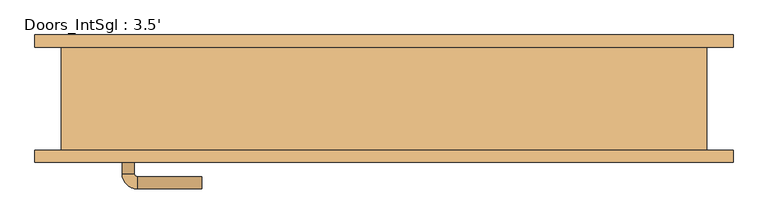
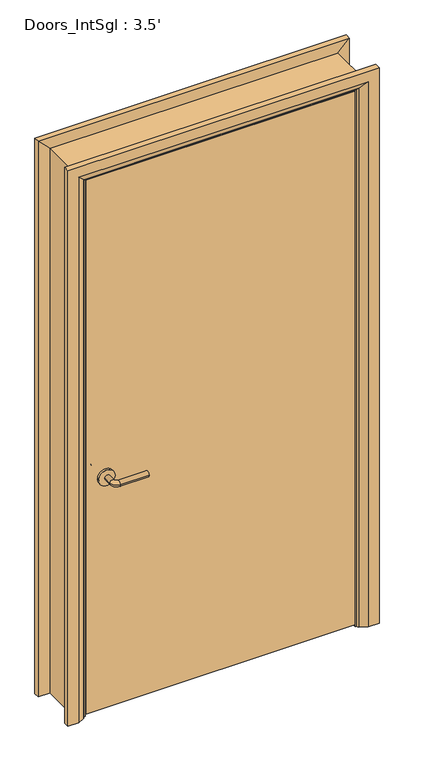
"""IFC4 building model written with IfcOpenShell, lengths in millimetres: door geometry, Doors_IntSgl : 3.5'."""

from ifc_helpers import new_model, si_unit, point, frame, frame_2d, origin, place, context, project, spatial, polyline, circle_curve, ellipse_curve, trimmed, segment, composite_curve, outline, extrude, faceted_brep, source, transform, mapped, element, save
from ifc_brep_helpers import plane_surface, cylinder_surface, revolved_surface, advanced_brep


def doors_intsgl_3_5_a4e1cc10(model_context):
    return source(origin(), model_context, "Body", "SolidModel", [
        advanced_brep(
        [(-426.4, -37.82, 900.0), (-406.4, -37.82, 900.0), (-426.4, -7.82, 900.0), (-406.4, -7.82, 900.0), (-401.4, -2.82, 900.0), (-401.4, 17.18, 900.0), (-296.4, 17.18, 900.0), (-296.4, -2.82, 900.0)],
        [
            (0, 1, circle_curve(frame((-416.4, -37.82, 900.0), z_axis=(0.0, -1.0, 0.0), x_axis=(1.0, 0.0, 0.0)), 10.0)),
            (1, 0, circle_curve(frame((-416.4, -37.82, 900.0), z_axis=(0.0, -1.0, 0.0), x_axis=(1.0, 0.0, 0.0)), 10.0)),
            (0, 2),
            (2, 3, circle_curve(frame((-416.4, -7.82, 900.0), z_axis=(0.0, -1.0, 0.0), x_axis=(1.0, 0.0, 0.0)), 10.0)),
            (3, 1),
            (3, 2, circle_curve(frame((-416.4, -7.82, 900.0), z_axis=(0.0, -1.0, 0.0), x_axis=(1.0, 0.0, 0.0)), 10.0)),
            (4, 3, circle_curve(frame((-401.4, -7.82, 900.0), z_axis=(0.0, 0.0, 1.0), x_axis=(-1.0, 0.0, 0.0)), 5.0)),
            (2, 5, circle_curve(frame((-401.4, -7.82, 900.0), z_axis=(0.0, 0.0, -1.0), x_axis=(-1.0, 0.0, 0.0)), 25.0)),
            (5, 4, circle_curve(frame((-401.4, 7.18, 900.0), z_axis=(-1.0, 0.0, 0.0), x_axis=(0.0, -1.0, 0.0)), 10.0)),
            (4, 5, circle_curve(frame((-401.4, 7.18, 900.0), z_axis=(-1.0, 0.0, 0.0), x_axis=(0.0, -1.0, 0.0)), 10.0)),
            (6, 7, circle_curve(frame((-296.4, 7.18, 900.0), z_axis=(1.0, 0.0, 0.0), x_axis=(0.0, -1.0, 0.0)), 10.0)),
            (7, 6, circle_curve(frame((-296.4, 7.18, 900.0), z_axis=(1.0, 0.0, 0.0), x_axis=(0.0, -1.0, 0.0)), 10.0)),
            (5, 6),
            (7, 4),
        ],
        [
            plane_surface(frame((-416.4, -37.82, 900.0), z_axis=(0.0, -1.0, 0.0), x_axis=(0.0, 0.0, 1.0))),
            cylinder_surface(frame((-416.4, -37.82, 900.0), z_axis=(0.0, -1.0, 0.0), x_axis=(1.0, 0.0, 0.0)), 10.0),
            revolved_surface(trimmed(ellipse_curve(frame((-416.4, -7.82, 900.0), z_axis=(0.0, -1.0, 0.0), x_axis=(1.0, 0.0, 0.0)), 10.0, 10.0), [point((-426.4, -7.82, 900.0))], [point((-406.4, -7.82, 900.0))], True, "CARTESIAN"), (-401.4, -7.82, 900.0), (0.0, 0.0, -1.0)),
            revolved_surface(trimmed(ellipse_curve(frame((-416.4, -7.82, 900.0), z_axis=(0.0, -1.0, 0.0), x_axis=(1.0, 0.0, 0.0)), 10.0, 10.0), [point((-406.4, -7.82, 900.0))], [point((-426.4, -7.82, 900.0))], True, "CARTESIAN"), (-401.4, -7.82, 900.0), (0.0, 0.0, -1.0)),
            plane_surface(frame((-296.4, 7.18, 900.0), z_axis=(1.0, 0.0, 0.0), x_axis=(0.0, 0.0, 1.0))),
            cylinder_surface(frame((-401.4, 7.18, 900.0), z_axis=(-1.0, 0.0, 0.0), x_axis=(0.0, -1.0, 0.0)), 10.0),
        ],
        [
            (0, [[1, 2]]),
            (1, [[-1, 3, 4, 5]]),
            (1, [[-2, -5, 6, -3]]),
            (2, [[7, -4, 8, 9]]),
            (3, [[-8, -6, -7, 10]]),
            (4, [[11, 12]]),
            (5, [[-9, 13, -12, 14]]),
            (5, [[-10, -14, -11, -13]]),
        ],
    ),
        extrude(outline(composite_curve([segment(trimmed(circle_curve(frame_2d((900.0, -418.9)), 30.0), [point((900.0, -448.9))], [point((900.0, -388.9))], False, "CARTESIAN"), True, "CONTINUOUS"), segment(trimmed(circle_curve(frame_2d((900.0, -418.9)), 30.0), [point((900.0, -388.9))], [point((900.0, -448.9))], False, "CARTESIAN"), True, "CONTINUOUS")], self_intersect=False)), frame((0.0, -45.82, 0.0), z_axis=(0.0, 1.0, 0.0), x_axis=(0.0, 0.0, 1.0)), (0.0, 0.0, 1.0), 8.0),
        advanced_brep(
        [(-426.4, -91.82, 900.0), (-406.4, -91.82, 900.0), (-406.4, -121.82, 900.0), (-426.4, -121.82, 900.0), (-401.4, -126.82, 900.0), (-401.4, -146.82, 900.0), (-296.4, -146.82, 900.0), (-296.4, -126.82, 900.0)],
        [
            (0, 1, circle_curve(frame((-416.4, -91.82, 900.0), z_axis=(0.0, 1.0, 0.0), x_axis=(1.0, 0.0, 0.0)), 10.0)),
            (1, 0, circle_curve(frame((-416.4, -91.82, 900.0), z_axis=(0.0, 1.0, 0.0), x_axis=(1.0, 0.0, 0.0)), 10.0)),
            (1, 2),
            (2, 3, circle_curve(frame((-416.4, -121.82, 900.0), z_axis=(0.0, 1.0, 0.0), x_axis=(1.0, 0.0, 0.0)), 10.0)),
            (3, 0),
            (3, 2, circle_curve(frame((-416.4, -121.82, 900.0), z_axis=(0.0, 1.0, 0.0), x_axis=(1.0, 0.0, 0.0)), 10.0)),
            (4, 5, circle_curve(frame((-401.4, -136.82, 900.0), z_axis=(-1.0, 0.0, 0.0), x_axis=(0.0, 1.0, 0.0)), 10.0)),
            (5, 3, circle_curve(frame((-401.4, -121.82, 900.0), z_axis=(0.0, 0.0, -1.0), x_axis=(-1.0, 0.0, 0.0)), 25.0)),
            (2, 4, circle_curve(frame((-401.4, -121.82, 900.0), z_axis=(0.0, 0.0, 1.0), x_axis=(-1.0, 0.0, 0.0)), 5.0)),
            (5, 4, circle_curve(frame((-401.4, -136.82, 900.0), z_axis=(-1.0, 0.0, 0.0), x_axis=(0.0, 1.0, 0.0)), 10.0)),
            (6, 7, circle_curve(frame((-296.4, -136.82, 900.0), z_axis=(1.0, 0.0, 0.0), x_axis=(0.0, 1.0, 0.0)), 10.0)),
            (7, 6, circle_curve(frame((-296.4, -136.82, 900.0), z_axis=(1.0, 0.0, 0.0), x_axis=(0.0, 1.0, 0.0)), 10.0)),
            (4, 7),
            (6, 5),
        ],
        [
            plane_surface(frame((-416.4, -91.82, 900.0), z_axis=(0.0, 1.0, 0.0), x_axis=(0.0, 0.0, 1.0))),
            cylinder_surface(frame((-416.4, -91.82, 900.0), z_axis=(0.0, 1.0, 0.0), x_axis=(1.0, 0.0, 0.0)), 10.0),
            revolved_surface(trimmed(ellipse_curve(frame((-416.4, -121.82, 900.0), z_axis=(0.0, -1.0, 0.0), x_axis=(1.0, 0.0, 0.0)), 10.0, 10.0), [point((-426.4, -121.82, 900.0))], [point((-406.4, -121.82, 900.0))], True, "CARTESIAN"), (-401.4, -121.82, 900.0), (0.0, 0.0, -1.0)),
            revolved_surface(trimmed(ellipse_curve(frame((-416.4, -121.82, 900.0), z_axis=(0.0, -1.0, 0.0), x_axis=(1.0, 0.0, 0.0)), 10.0, 10.0), [point((-406.4, -121.82, 900.0))], [point((-426.4, -121.82, 900.0))], True, "CARTESIAN"), (-401.4, -121.82, 900.0), (0.0, 0.0, -1.0)),
            plane_surface(frame((-296.4, -136.82, 900.0), z_axis=(1.0, 0.0, 0.0), x_axis=(0.0, 0.0, 1.0))),
            cylinder_surface(frame((-401.4, -136.82, 900.0), z_axis=(-1.0, 0.0, 0.0), x_axis=(0.0, 1.0, 0.0)), 10.0),
        ],
        [
            (0, [[1, 2]]),
            (1, [[3, 4, 5, -2]]),
            (1, [[-5, 6, -3, -1]]),
            (2, [[7, 8, -4, 9]]),
            (3, [[10, -9, -6, -8]]),
            (4, [[11, 12]]),
            (5, [[13, -11, 14, -7]]),
            (5, [[-14, -12, -13, -10]]),
        ],
    ),
        extrude(outline(composite_curve([segment(trimmed(circle_curve(frame_2d((900.0, -418.9)), 30.0), [point((900.0, -448.9))], [point((900.0, -388.9))], False, "CARTESIAN"), True, "CONTINUOUS"), segment(trimmed(circle_curve(frame_2d((900.0, -418.9)), 30.0), [point((900.0, -388.9))], [point((900.0, -448.9))], False, "CARTESIAN"), True, "CONTINUOUS")], self_intersect=False)), frame((0.0, -91.82, 0.0), z_axis=(0.0, 1.0, 0.0), x_axis=(0.0, 0.0, 1.0)), (0.0, 0.0, 1.0), 8.0),
        extrude(outline(polyline([(491.4, -45.82), (491.4, -83.82), (-491.4, -83.82), (-491.4, -45.82), (491.4, -45.82)])), frame((0.0, 0.0, 8.0), z_axis=(0.0, 0.0, 1.0), x_axis=(1.0, 0.0, 0.0)), (0.0, 0.0, 1.0), 2060.0),
        advanced_brep(
        [(568.4, -103.82, 0.0), (528.4, -103.82, 0.0), (502.4, -89.82, 0.0), (498.4, -83.82, 0.0), (568.4, -83.82, 0.0), (568.4, -83.82, 2145.0), (568.4, -103.82, 2145.0), (498.4, -83.82, 2075.0), (-498.4, -83.82, 2075.0), (-498.4, -83.82, 0.0), (-568.4, -83.82, 0.0), (-568.4, -83.82, 2145.0), (502.4, -89.82, 2079.0), (528.4, -103.82, 2105.0), (-568.4, -103.82, 2145.0), (-568.4, -103.82, 0.0), (-528.4, -103.82, 0.0), (-528.4, -103.82, 2105.0), (-502.4, -89.82, 0.0), (-502.4, -89.82, 2079.0)],
        [
            (0, 1),
            (1, 2),
            (2, 3, circle_curve(frame((506.4, -82.82, 0.0), z_axis=(0.0, 0.0, -1.0), x_axis=(1.0, 0.0, 0.0)), 8.0622577)),
            (3, 4),
            (4, 0),
            (4, 5),
            (5, 6),
            (6, 0),
            (3, 7),
            (7, 8),
            (8, 9),
            (9, 10),
            (10, 11),
            (11, 5),
            (2, 12),
            (12, 7, ellipse_curve(frame((506.4, -82.82, 2083.0), z_axis=(0.7071067811865475, 0.0, -0.7071067811865475), x_axis=(-0.7071067811865474, 0.0, -0.7071067811865476)), 11.4017543, 8.0622577)),
            (1, 13),
            (13, 12),
            (6, 14),
            (14, 15),
            (15, 16),
            (16, 17),
            (17, 13),
            (10, 15),
            (14, 11),
            (9, 18, circle_curve(frame((-506.4, -82.82, 0.0), z_axis=(0.0, 0.0, -1.0), x_axis=(-1.0, 0.0, 0.0)), 8.0622577)),
            (18, 16),
            (19, 18),
            (8, 19, ellipse_curve(frame((-506.4, -82.82, 2083.0), z_axis=(-0.7071067811865475, 0.0, -0.7071067811865475), x_axis=(-0.7071067811865474, 0.0, 0.7071067811865476)), 11.4017543, 8.0622577)),
            (19, 17),
            (12, 19),
        ],
        [
            plane_surface(frame((498.4, -83.82, 0.0), z_axis=(0.0, 0.0, -1.0), x_axis=(0.0, 1.0, 0.0))),
            plane_surface(frame((568.4, -103.82, 0.0), z_axis=(1.0, 0.0, 0.0), x_axis=(0.0, 0.0, 1.0))),
            plane_surface(frame((568.4, -83.82, 0.0), z_axis=(0.0, 1.0, 0.0), x_axis=(0.0, 0.0, 1.0))),
            cylinder_surface(frame((506.4, -82.82, 0.0), z_axis=(0.0, 0.0, -1.0), x_axis=(1.0, 0.0, 0.0)), 8.0622577),
            plane_surface(frame((502.4, -89.82, 0.0), z_axis=(-0.4740998230350126, -0.880471099922178, 0.0), x_axis=(0.0, 0.0, 1.0))),
            plane_surface(frame((528.4, -103.82, 0.0), z_axis=(0.0, -1.0, 0.0), x_axis=(0.0, 0.0, 1.0))),
            plane_surface(frame((-568.4, -103.82, 2145.0), z_axis=(-1.0, 0.0, 0.0), x_axis=(0.0, 0.0, -1.0))),
            plane_surface(frame((-498.4, -83.82, 0.0), z_axis=(0.0, 0.0, -1.0), x_axis=(0.0, 1.0, 0.0))),
            cylinder_surface(frame((-506.4, -82.82, 2075.0), z_axis=(0.0, 0.0, 1.0), x_axis=(-1.0, 0.0, 0.0)), 8.0622577),
            plane_surface(frame((-502.4, -89.82, 2079.0), z_axis=(0.47409982303501824, -0.8804710999221749, 0.0), x_axis=(0.0, 0.0, -1.0))),
            plane_surface(frame((568.4, -103.82, 2145.0), z_axis=(0.0, 0.0, 1.0), x_axis=(-1.0, 0.0, 0.0))),
            cylinder_surface(frame((498.4, -82.82, 2083.0), z_axis=(1.0, 0.0, 0.0), x_axis=(0.0, 0.0, 1.0)), 8.0622577),
            plane_surface(frame((502.4, -89.82, 2079.0), z_axis=(0.0, -0.8804710999221764, -0.4740998230350154), x_axis=(-1.0, 0.0, 0.0))),
        ],
        [
            (0, [[1, 2, 3, 4, 5]]),
            (1, [[6, 7, 8, -5]]),
            (2, [[9, 10, 11, 12, 13, 14, -6, -4]]),
            (3, [[15, 16, -9, -3]]),
            (4, [[17, 18, -15, -2]]),
            (5, [[-8, 19, 20, 21, 22, 23, -17, -1]]),
            (6, [[-13, 24, -20, 25]]),
            (7, [[-24, -12, 26, 27, -21]]),
            (8, [[28, -26, -11, 29]]),
            (9, [[-22, -27, -28, 30]]),
            (10, [[-14, -25, -19, -7]]),
            (11, [[31, -29, -10, -16]]),
            (12, [[-23, -30, -31, -18]]),
        ],
    ),
        extrude(outline(polyline([(0.0, -474.4), (2051.0, -474.4), (2051.0, 474.4), (0.0, 474.4), (0.0, 493.4), (2070.0, 493.4), (2070.0, -493.4), (0.0, -493.4), (0.0, -474.4)])), frame((0.0, -43.82, 0.0), z_axis=(0.0, 1.0, 0.0), x_axis=(0.0, 0.0, 1.0)), (0.0, 0.0, 1.0), 32.0),
        advanced_brep(
        [(-568.4, 103.82, 0.0), (-528.4, 103.82, 0.0), (-502.4, 89.82, 0.0), (-498.4, 83.82, 0.0), (-568.4, 83.82, 0.0), (-568.4, 83.82, 2145.0), (-568.4, 103.82, 2145.0), (-498.4, 83.82, 2075.0), (-502.4, 89.82, 2079.0), (-528.4, 103.82, 2105.0), (568.4, 103.82, 0.0), (568.4, 83.82, 0.0), (498.4, 83.82, 0.0), (502.4, 89.82, 0.0), (528.4, 103.82, 0.0), (568.4, 103.82, 2145.0), (528.4, 103.82, 2105.0), (502.4, 89.82, 2079.0), (498.4, 83.82, 2075.0), (568.4, 83.82, 2145.0)],
        [
            (0, 1),
            (1, 2),
            (2, 3, circle_curve(frame((-506.4, 82.82, 0.0), z_axis=(0.0, 0.0, -1.0), x_axis=(-1.0, 0.0, 0.0)), 8.0622577)),
            (3, 4),
            (4, 0),
            (4, 5),
            (5, 6),
            (6, 0),
            (3, 7),
            (7, 5),
            (2, 8),
            (8, 7, ellipse_curve(frame((-506.4, 82.82, 2083.0), z_axis=(-0.7071067811865475, 0.0, -0.7071067811865475), x_axis=(0.7071067811865474, 0.0, -0.7071067811865476)), 11.4017543, 8.0622577)),
            (1, 9),
            (9, 8),
            (6, 9),
            (10, 11),
            (11, 12),
            (12, 13, circle_curve(frame((506.4, 82.82, 0.0), z_axis=(0.0, 0.0, -1.0), x_axis=(1.0, 0.0, 0.0)), 8.0622577)),
            (13, 14),
            (14, 10),
            (15, 10),
            (14, 16),
            (16, 15),
            (13, 17),
            (17, 16),
            (12, 18),
            (18, 17, ellipse_curve(frame((506.4, 82.82, 2083.0), z_axis=(0.7071067811865475, 0.0, -0.7071067811865475), x_axis=(0.7071067811865474, 0.0, 0.7071067811865476)), 11.4017543, 8.0622577)),
            (11, 19),
            (19, 18),
            (15, 19),
            (5, 19),
            (15, 6),
            (7, 18),
            (8, 17),
            (9, 16),
        ],
        [
            plane_surface(frame((-498.4, 156.6210989, 0.0), z_axis=(0.0, 0.0, -1.0), x_axis=(1.0, 0.0, 0.0))),
            plane_surface(frame((-568.4, 103.82, 0.0), z_axis=(-1.0, 0.0, 0.0), x_axis=(0.0, 0.0, 1.0))),
            plane_surface(frame((-568.4, 83.82, 0.0), z_axis=(0.0, -1.0, 0.0), x_axis=(0.0, 0.0, 1.0))),
            cylinder_surface(frame((-506.4, 82.82, 0.0), z_axis=(0.0, 0.0, -1.0), x_axis=(-1.0, 0.0, 0.0)), 8.0622577),
            plane_surface(frame((-502.4, 89.82, 0.0), z_axis=(0.4740998230350183, 0.8804710999221749, 0.0), x_axis=(0.0, 0.0, 1.0))),
            plane_surface(frame((-528.4, 103.82, 0.0), z_axis=(0.0, 1.0, 0.0), x_axis=(0.0, 0.0, 1.0))),
            plane_surface(frame((498.4, 156.6210989, 0.0), z_axis=(0.0, 0.0, -1.0), x_axis=(-1.0, 0.0, 0.0))),
            plane_surface(frame((528.4, 103.82, 2105.0), z_axis=(0.0, 1.0, 0.0), x_axis=(0.0, 0.0, -1.0))),
            plane_surface(frame((502.4, 89.82, 2079.0), z_axis=(-0.4740998230350183, 0.8804710999221749, 0.0), x_axis=(0.0, 0.0, -1.0))),
            cylinder_surface(frame((506.4, 82.82, 2075.0), z_axis=(0.0, 0.0, 1.0), x_axis=(1.0, 0.0, 0.0)), 8.0622577),
            plane_surface(frame((568.4, 83.82, 2145.0), z_axis=(0.0, -1.0, 0.0), x_axis=(0.0, 0.0, -1.0))),
            plane_surface(frame((568.4, 103.82, 2145.0), z_axis=(1.0, 0.0, 0.0), x_axis=(0.0, 0.0, -1.0))),
            plane_surface(frame((-568.4, 103.82, 2145.0), z_axis=(0.0, 0.0, 1.0), x_axis=(1.0, 0.0, 0.0))),
            plane_surface(frame((-568.4, 83.82, 2145.0), z_axis=(0.0, -1.0, 0.0), x_axis=(1.0, 0.0, 0.0))),
            cylinder_surface(frame((-498.4, 82.82, 2083.0), z_axis=(-1.0, 0.0, 0.0), x_axis=(0.0, 0.0, 1.0)), 8.0622577),
            plane_surface(frame((-502.4, 89.82, 2079.0), z_axis=(0.0, 0.8804710999221749, -0.4740998230350183), x_axis=(1.0, 0.0, 0.0))),
            plane_surface(frame((-528.4, 103.82, 2105.0), z_axis=(0.0, 1.0, 0.0), x_axis=(1.0, 0.0, 0.0))),
        ],
        [
            (0, [[1, 2, 3, 4, 5]]),
            (1, [[6, 7, 8, -5]]),
            (2, [[9, 10, -6, -4]]),
            (3, [[11, 12, -9, -3]]),
            (4, [[13, 14, -11, -2]]),
            (5, [[-8, 15, -13, -1]]),
            (6, [[16, 17, 18, 19, 20]]),
            (7, [[21, -20, 22, 23]]),
            (8, [[-22, -19, 24, 25]]),
            (9, [[-24, -18, 26, 27]]),
            (10, [[-26, -17, 28, 29]]),
            (11, [[-28, -16, -21, 30]]),
            (12, [[31, -30, 32, -7]]),
            (13, [[33, -29, -31, -10]]),
            (14, [[34, -27, -33, -12]]),
            (15, [[35, -25, -34, -14]]),
            (16, [[-32, -23, -35, -15]]),
        ],
    ),
        faceted_brep([(-493.4, -83.82, 0.0), (-525.4, -83.82, 0.0), (-525.4, 83.82, 0.0), (-493.4, 83.82, 0.0), (-493.4, 83.82, 2070.0), (-493.4, -83.82, 2070.0), (-525.4, 83.82, 2102.0), (-525.4, -83.82, 2102.0), (493.4, -83.82, 0.0), (493.4, 83.82, 0.0), (525.4, 83.82, 0.0), (525.4, -83.82, 0.0), (493.4, -83.82, 2070.0), (525.4, -83.82, 2102.0), (525.4, 83.82, 2102.0), (493.4, 83.82, 2070.0)], [[[0, 1, 2, 3]], [[3, 4, 5, 0]], [[2, 6, 4, 3]], [[1, 7, 6, 2]], [[0, 5, 7, 1]], [[8, 9, 10, 11]], [[12, 8, 11, 13]], [[13, 11, 10, 14]], [[14, 10, 9, 15]], [[15, 9, 8, 12]], [[4, 15, 12, 5]], [[6, 14, 15, 4]], [[7, 13, 14, 6]], [[5, 12, 13, 7]]]),
    ])


if __name__ == "__main__":
    model = new_model("IFC4")
    model_context = context("Model", 3, world=origin())
    ifc_project = project(units=[si_unit("LENGTHUNIT", "METRE", prefix="MILLI")], contexts=[model_context])
    site = spatial("IfcSite", under=ifc_project)
    building = spatial("IfcBuilding", under=site)
    placement = place(None, origin())
    doors_intsgl_3_5_shape = doors_intsgl_3_5_a4e1cc10(model_context)
    element("IfcDoor", 1, ObjectType="Doors_IntSgl : 3.5'", at=placement, inside=building, context=model_context, shape_type="MappedRepresentation", body=[
        mapped(doors_intsgl_3_5_shape, transform((0.0, 0.0, 0.0), x_axis=(1.0, 0.0, 0.0), y_axis=(0.0, 1.0, 0.0), z_axis=(0.0, 0.0, 1.0))),
    ])
    save(model, "model.ifc")

# Revit data of these elements
# Type "Doors_IntSgl : 3.5'"
#   Type Mark = "51"
#   Type Comments = "Internal Single"
#   Operation = "SingleSwingRight"
#   Manufacturer = "Revit"
#   Keynote = "L20"
#   Description = "Internal Single Door"
#   Analytic Construction = "Metal"
#   UnderCut = 0.026247 ft
#   Tolerance = 0.006562 ft
#   Thickness = 0.124672 ft
#   Thermal Resistance (R) = 0.270117 (m²·K)/W
#   Structural Tolerance = 0.026247 ft
#   StopDepth = 0.104987 ft
#   Stop Thickness = 0.062336 ft
#   Rough Width = 3.5 ft
#   Rough Height = 6.922572 ft
#   Height to Top Lock Rail = 3.28084 ft
#   Heat Transfer Coefficient (U) = 3.7021 W/(m²·K)
#   Handle Z Distance = 2.952756 ft
#   Handle X Distance = 0.246063 ft
#   Frame Thickness = 0.104987 ft
#   Door Panel Width = 3.224409 ft
#   Door Panel Thickness = 0.124672 ft
#   Door Panel Offset = 0.0 ft
#   Height = 6.922572 ft
#   Width = 3.5 ft
#   Door Panel Height = 6.75853 ft
#   Architrave Setback = 0.016404 ft
#   Vis - Ironmongery = yes
#   Material Ironmongery = Door - Handle
#   Material Frame = Door - Frame/Mullion (1)
#   Material Door = Door - Panel
#   Material Architrave = Door - Architrave
#   Visual Light Transmittance = 0
#   Solar Heat Gain Coefficient = 0
#   Function = (empty or 0)
#   Wall Closure = (empty or 0)
# Element 1 (IfcDoor, "Doors_IntSgl : 3.5'")
#   Materials on its faces: "Door - Architrave", "Door - Handle", "Door - Frame/Mullion (1)", "Door - Panel"
# Materials
#   "Door - Handle": colour RGB 0 0 0, transparency 0, Keynote = "P21", Cost = 0
#   "Door - Frame/Mullion (1)": class "Wood", colour RGB 212 179 113, transparency 0, Keynote = "L20", Cost = 0
#   "Door - Panel": class "Wood", colour RGB 210 159 95, transparency 0, Keynote = "L20", Cost = 0
#   "Door - Architrave": class "Wood", colour RGB 154 90 5, transparency 0, Keynote = "P20", Cost = 0
